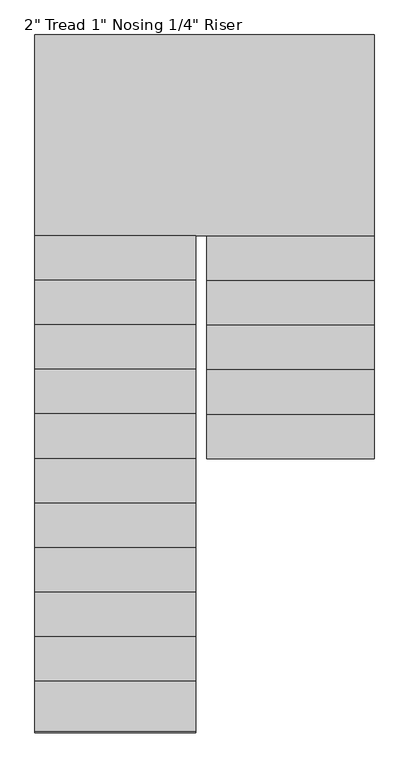
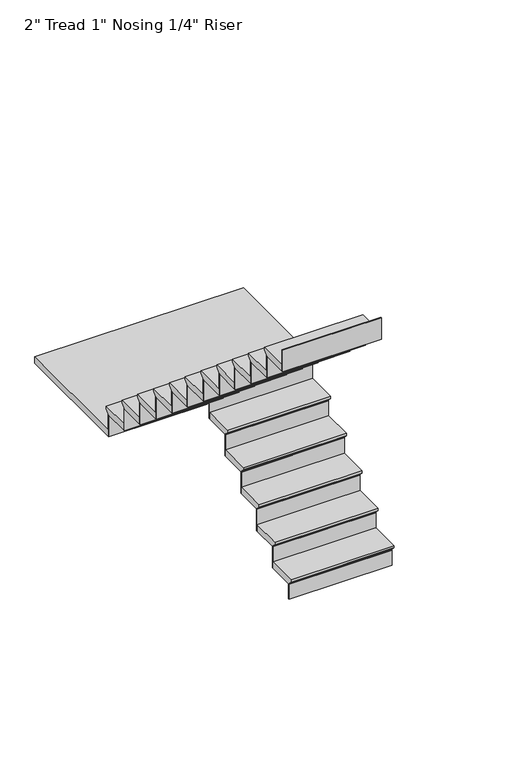
"""IFC4 building model written with IfcOpenShell, lengths in millimetres: stair flight geometry."""

from ifc_helpers import new_model, si_unit, origin, place, context, project, spatial, faceted_brep, source, transform, mapped, element, save


def stair_flight_e7bd6350(model_context):
    return source(origin(), model_context, "Body", "Brep", [
        faceted_brep([(-3749.597125, 2714.6319226, 30477.8833333), (-3749.597125, 2714.6319226, 30496.9333333), (-4512.2136682, 2714.6319226, 30496.9333333), (-4512.2136682, 2714.6319226, 30477.8833333), (-3749.597125, 2740.0319226, 30452.4833333), (-4512.2136682, 2740.0319226, 30452.4833333), (-3749.597125, 2943.2319226, 30496.9333333), (-4512.2136682, 2943.2319226, 30496.9333333), (-4512.2136682, 2740.0319226, 30446.1333333), (-4512.2136682, 2943.2319226, 30446.1333333), (-3749.597125, 2943.2319226, 30446.1333333), (-3749.597125, 2740.0319226, 30446.1333333)], [[[0, 1, 2, 3]], [[4, 0, 3, 5]], [[2, 1, 6, 7]], [[8, 9, 10, 11]], [[2, 7, 9, 8, 5, 3]], [[8, 11, 4, 5]], [[6, 1, 0, 4, 11, 10]], [[7, 6, 10, 9]]]),
        faceted_brep([(-3749.597125, 2740.0319226, 30446.1333333), (-3749.597125, 2740.0319226, 30327.6), (-3749.597125, 2746.3819226, 30327.6), (-3749.597125, 2746.3819226, 30446.1333333), (-4512.2136682, 2740.0319226, 30446.1333333), (-4512.2136682, 2746.3819226, 30446.1333333), (-4512.2136682, 2746.3819226, 30327.6), (-4512.2136682, 2740.0319226, 30327.6)], [[[0, 1, 2, 3]], [[4, 5, 6, 7]], [[1, 0, 4, 7]], [[2, 1, 7, 6]], [[3, 2, 6, 5]], [[0, 3, 5, 4]]]),
        faceted_brep([(-3749.597125, 2943.2319226, 30615.4666667), (-3749.597125, 2943.2319226, 30446.1333333), (-3749.597125, 2949.5819226, 30446.1333333), (-3749.597125, 2949.5819226, 30615.4666667), (-4512.2136682, 2943.2319226, 30615.4666667), (-4512.2136682, 2949.5819226, 30615.4666667), (-4512.2136682, 2949.5819226, 30446.1333333), (-4512.2136682, 2943.2319226, 30446.1333333)], [[[0, 1, 2, 3]], [[4, 5, 6, 7]], [[1, 0, 4, 7]], [[2, 1, 7, 6]], [[3, 2, 6, 5]], [[0, 3, 5, 4]]]),
        faceted_brep([(-4512.2136682, 2917.8319226, 30666.2666667), (-3749.597125, 2917.8319226, 30666.2666667), (-3749.597125, 3146.4319226, 30666.2666667), (-4512.2136682, 3146.4319226, 30666.2666667), (-4512.2136682, 2943.2319226, 30615.4666667), (-4512.2136682, 3146.4319226, 30615.4666667), (-3749.597125, 3146.4319226, 30615.4666667), (-3749.597125, 2943.2319226, 30615.4666667), (-4512.2136682, 2943.2319226, 30621.8166667), (-4512.2136682, 2917.8319226, 30647.2166667), (-3749.597125, 2943.2319226, 30621.8166667), (-3749.597125, 2917.8319226, 30647.2166667)], [[[0, 1, 2, 3]], [[4, 5, 6, 7]], [[0, 3, 5, 4, 8, 9]], [[4, 7, 10, 8]], [[2, 1, 11, 10, 7, 6]], [[3, 2, 6, 5]], [[11, 1, 0, 9]], [[10, 11, 9, 8]]]),
        faceted_brep([(-3749.597125, 3146.4319226, 30784.8), (-3749.597125, 3146.4319226, 30615.4666667), (-3749.597125, 3152.7819226, 30615.4666667), (-3749.597125, 3152.7819226, 30784.8), (-4512.2136682, 3146.4319226, 30784.8), (-4512.2136682, 3152.7819226, 30784.8), (-4512.2136682, 3152.7819226, 30615.4666667), (-4512.2136682, 3146.4319226, 30615.4666667)], [[[0, 1, 2, 3]], [[4, 5, 6, 7]], [[1, 0, 4, 7]], [[2, 1, 7, 6]], [[3, 2, 6, 5]], [[0, 3, 5, 4]]]),
        faceted_brep([(-4512.2136682, 3121.0319226, 30835.6), (-3749.597125, 3121.0319226, 30835.6), (-3749.597125, 3349.6319226, 30835.6), (-4512.2136682, 3349.6319226, 30835.6), (-4512.2136682, 3146.4319226, 30784.8), (-4512.2136682, 3349.6319226, 30784.8), (-3749.597125, 3349.6319226, 30784.8), (-3749.597125, 3146.4319226, 30784.8), (-4512.2136682, 3146.4319226, 30791.15), (-4512.2136682, 3121.0319226, 30816.55), (-3749.597125, 3146.4319226, 30791.15), (-3749.597125, 3121.0319226, 30816.55)], [[[0, 1, 2, 3]], [[4, 5, 6, 7]], [[0, 3, 5, 4, 8, 9]], [[4, 7, 10, 8]], [[2, 1, 11, 10, 7, 6]], [[3, 2, 6, 5]], [[11, 1, 0, 9]], [[10, 11, 9, 8]]]),
        faceted_brep([(-3749.597125, 3349.6319226, 30954.1333333), (-3749.597125, 3349.6319226, 30784.8), (-3749.597125, 3355.9819226, 30784.8), (-3749.597125, 3355.9819226, 30954.1333333), (-4512.2136682, 3349.6319226, 30954.1333333), (-4512.2136682, 3355.9819226, 30954.1333333), (-4512.2136682, 3355.9819226, 30784.8), (-4512.2136682, 3349.6319226, 30784.8)], [[[0, 1, 2, 3]], [[4, 5, 6, 7]], [[1, 0, 4, 7]], [[2, 1, 7, 6]], [[3, 2, 6, 5]], [[0, 3, 5, 4]]]),
        faceted_brep([(-4512.2136682, 3324.2319226, 31004.9333333), (-3749.597125, 3324.2319226, 31004.9333333), (-3749.597125, 3552.8319226, 31004.9333333), (-4512.2136682, 3552.8319226, 31004.9333333), (-4512.2136682, 3349.6319226, 30954.1333333), (-4512.2136682, 3552.8319226, 30954.1333333), (-3749.597125, 3552.8319226, 30954.1333333), (-3749.597125, 3349.6319226, 30954.1333333), (-4512.2136682, 3349.6319226, 30960.4833333), (-4512.2136682, 3324.2319226, 30985.8833333), (-3749.597125, 3349.6319226, 30960.4833333), (-3749.597125, 3324.2319226, 30985.8833333)], [[[0, 1, 2, 3]], [[4, 5, 6, 7]], [[0, 3, 5, 4, 8, 9]], [[4, 7, 10, 8]], [[2, 1, 11, 10, 7, 6]], [[3, 2, 6, 5]], [[11, 1, 0, 9]], [[10, 11, 9, 8]]]),
        faceted_brep([(-3749.597125, 3552.8319226, 31123.4666667), (-3749.597125, 3552.8319226, 30954.1333333), (-3749.597125, 3559.1819226, 30954.1333333), (-3749.597125, 3559.1819226, 31123.4666667), (-4512.2136682, 3552.8319226, 31123.4666667), (-4512.2136682, 3559.1819226, 31123.4666667), (-4512.2136682, 3559.1819226, 30954.1333333), (-4512.2136682, 3552.8319226, 30954.1333333)], [[[0, 1, 2, 3]], [[4, 5, 6, 7]], [[1, 0, 4, 7]], [[2, 1, 7, 6]], [[3, 2, 6, 5]], [[0, 3, 5, 4]]]),
        faceted_brep([(-4512.2136682, 3527.4319226, 31174.2666667), (-3749.597125, 3527.4319226, 31174.2666667), (-3749.597125, 3756.0319226, 31174.2666667), (-4512.2136682, 3756.0319226, 31174.2666667), (-4512.2136682, 3552.8319226, 31123.4666667), (-4512.2136682, 3756.0319226, 31123.4666667), (-3749.597125, 3756.0319226, 31123.4666667), (-3749.597125, 3552.8319226, 31123.4666667), (-4512.2136682, 3552.8319226, 31129.8166667), (-4512.2136682, 3527.4319226, 31155.2166667), (-3749.597125, 3552.8319226, 31129.8166667), (-3749.597125, 3527.4319226, 31155.2166667)], [[[0, 1, 2, 3]], [[4, 5, 6, 7]], [[0, 3, 5, 4, 8, 9]], [[4, 7, 10, 8]], [[2, 1, 11, 10, 7, 6]], [[3, 2, 6, 5]], [[11, 1, 0, 9]], [[10, 11, 9, 8]]]),
        faceted_brep([(-3749.597125, 3756.0319226, 31292.8), (-3749.597125, 3756.0319226, 31123.4666667), (-3749.597125, 3762.3819226, 31123.4666667), (-3749.597125, 3762.3819226, 31292.8), (-4512.2136682, 3756.0319226, 31292.8), (-4512.2136682, 3762.3819226, 31292.8), (-4512.2136682, 3762.3819226, 31123.4666667), (-4512.2136682, 3756.0319226, 31123.4666667)], [[[0, 1, 2, 3]], [[4, 5, 6, 7]], [[1, 0, 4, 7]], [[2, 1, 7, 6]], [[3, 2, 6, 5]], [[0, 3, 5, 4]]]),
        faceted_brep([(-4563.0136682, 3705.2319226, 31343.6), (-4563.0136682, 3730.6319226, 31343.6), (-3749.597125, 3730.6319226, 31343.6), (-3749.597125, 4645.0319226, 31343.6), (-5295.0246464, 4645.0319226, 31343.6), (-5295.0246464, 3705.2319226, 31343.6), (-4563.0136682, 3730.6319226, 31292.8), (-4563.0136682, 3705.2319226, 31292.8), (-5295.0246464, 3705.2319226, 31292.8), (-5295.0246464, 4645.0319226, 31292.8), (-3749.597125, 4645.0319226, 31292.8), (-3749.597125, 3756.0319226, 31292.8), (-4512.2136682, 3756.0319226, 31292.8), (-4512.2136682, 3730.6319226, 31292.8), (-4512.2136682, 3730.6319226, 31324.55), (-3749.597125, 3730.6319226, 31324.55), (-4512.2136682, 3756.0319226, 31299.15), (-3749.597125, 3756.0319226, 31299.15)], [[[0, 1, 2, 3, 4, 5]], [[6, 7, 8, 9, 10, 11, 12, 13]], [[1, 0, 7, 6]], [[2, 1, 6, 13, 14, 15]], [[13, 12, 16, 14]], [[12, 11, 17, 16]], [[3, 2, 15, 17, 11, 10]], [[4, 3, 10, 9]], [[5, 4, 9, 8]], [[0, 5, 8, 7]], [[17, 15, 14, 16]]]),
        faceted_brep([(-5295.0246464, 3705.2319226, 31462.1333333), (-5295.0246464, 3705.2319226, 31292.8), (-5295.0246464, 3698.8819226, 31292.8), (-5295.0246464, 3698.8819226, 31462.1333333), (-4563.0136682, 3705.2319226, 31462.1333333), (-4563.0136682, 3698.8819226, 31462.1333333), (-4563.0136682, 3698.8819226, 31292.8), (-4563.0136682, 3705.2319226, 31292.8)], [[[0, 1, 2, 3]], [[4, 5, 6, 7]], [[1, 0, 4, 7]], [[2, 1, 7, 6]], [[3, 2, 6, 5]], [[0, 3, 5, 4]]]),
        faceted_brep([(-4563.0136682, 3730.6319226, 31512.9333333), (-5295.0246464, 3730.6319226, 31512.9333333), (-5295.0246464, 3502.0319226, 31512.9333333), (-4563.0136682, 3502.0319226, 31512.9333333), (-4563.0136682, 3705.2319226, 31462.1333333), (-4563.0136682, 3502.0319226, 31462.1333333), (-5295.0246464, 3502.0319226, 31462.1333333), (-5295.0246464, 3705.2319226, 31462.1333333), (-4563.0136682, 3705.2319226, 31468.4833333), (-4563.0136682, 3730.6319226, 31493.8833333), (-5295.0246464, 3705.2319226, 31468.4833333), (-5295.0246464, 3730.6319226, 31493.8833333)], [[[0, 1, 2, 3]], [[4, 5, 6, 7]], [[0, 3, 5, 4, 8, 9]], [[4, 7, 10, 8]], [[2, 1, 11, 10, 7, 6]], [[3, 2, 6, 5]], [[11, 1, 0, 9]], [[10, 11, 9, 8]]]),
        faceted_brep([(-5295.0246464, 3502.0319226, 31631.4666667), (-5295.0246464, 3502.0319226, 31462.1333333), (-5295.0246464, 3495.6819226, 31462.1333333), (-5295.0246464, 3495.6819226, 31631.4666667), (-4563.0136682, 3502.0319226, 31631.4666667), (-4563.0136682, 3495.6819226, 31631.4666667), (-4563.0136682, 3495.6819226, 31462.1333333), (-4563.0136682, 3502.0319226, 31462.1333333)], [[[0, 1, 2, 3]], [[4, 5, 6, 7]], [[1, 0, 4, 7]], [[2, 1, 7, 6]], [[3, 2, 6, 5]], [[0, 3, 5, 4]]]),
        faceted_brep([(-4563.0136682, 3527.4319226, 31682.2666667), (-5295.0246464, 3527.4319226, 31682.2666667), (-5295.0246464, 3298.8319226, 31682.2666667), (-4563.0136682, 3298.8319226, 31682.2666667), (-4563.0136682, 3502.0319226, 31631.4666667), (-4563.0136682, 3298.8319226, 31631.4666667), (-5295.0246464, 3298.8319226, 31631.4666667), (-5295.0246464, 3502.0319226, 31631.4666667), (-4563.0136682, 3502.0319226, 31637.8166667), (-4563.0136682, 3527.4319226, 31663.2166667), (-5295.0246464, 3502.0319226, 31637.8166667), (-5295.0246464, 3527.4319226, 31663.2166667)], [[[0, 1, 2, 3]], [[4, 5, 6, 7]], [[0, 3, 5, 4, 8, 9]], [[4, 7, 10, 8]], [[2, 1, 11, 10, 7, 6]], [[3, 2, 6, 5]], [[11, 1, 0, 9]], [[10, 11, 9, 8]]]),
        faceted_brep([(-5295.0246464, 3298.8319226, 31800.8), (-5295.0246464, 3298.8319226, 31631.4666667), (-5295.0246464, 3292.4819226, 31631.4666667), (-5295.0246464, 3292.4819226, 31800.8), (-4563.0136682, 3298.8319226, 31800.8), (-4563.0136682, 3292.4819226, 31800.8), (-4563.0136682, 3292.4819226, 31631.4666667), (-4563.0136682, 3298.8319226, 31631.4666667)], [[[0, 1, 2, 3]], [[4, 5, 6, 7]], [[1, 0, 4, 7]], [[2, 1, 7, 6]], [[3, 2, 6, 5]], [[0, 3, 5, 4]]]),
        faceted_brep([(-4563.0136682, 3324.2319226, 31851.6), (-5295.0246464, 3324.2319226, 31851.6), (-5295.0246464, 3095.6319226, 31851.6), (-4563.0136682, 3095.6319226, 31851.6), (-4563.0136682, 3298.8319226, 31800.8), (-4563.0136682, 3095.6319226, 31800.8), (-5295.0246464, 3095.6319226, 31800.8), (-5295.0246464, 3298.8319226, 31800.8), (-4563.0136682, 3298.8319226, 31807.15), (-4563.0136682, 3324.2319226, 31832.55), (-5295.0246464, 3298.8319226, 31807.15), (-5295.0246464, 3324.2319226, 31832.55)], [[[0, 1, 2, 3]], [[4, 5, 6, 7]], [[0, 3, 5, 4, 8, 9]], [[4, 7, 10, 8]], [[2, 1, 11, 10, 7, 6]], [[3, 2, 6, 5]], [[11, 1, 0, 9]], [[10, 11, 9, 8]]]),
        faceted_brep([(-5295.0246464, 3095.6319226, 31970.1333333), (-5295.0246464, 3095.6319226, 31800.8), (-5295.0246464, 3089.2819226, 31800.8), (-5295.0246464, 3089.2819226, 31970.1333333), (-4563.0136682, 3095.6319226, 31970.1333333), (-4563.0136682, 3089.2819226, 31970.1333333), (-4563.0136682, 3089.2819226, 31800.8), (-4563.0136682, 3095.6319226, 31800.8)], [[[0, 1, 2, 3]], [[4, 5, 6, 7]], [[1, 0, 4, 7]], [[2, 1, 7, 6]], [[3, 2, 6, 5]], [[0, 3, 5, 4]]]),
        faceted_brep([(-4563.0136682, 3121.0319226, 32020.9333333), (-5295.0246464, 3121.0319226, 32020.9333333), (-5295.0246464, 2892.4319226, 32020.9333333), (-4563.0136682, 2892.4319226, 32020.9333333), (-4563.0136682, 3095.6319226, 31970.1333333), (-4563.0136682, 2892.4319226, 31970.1333333), (-5295.0246464, 2892.4319226, 31970.1333333), (-5295.0246464, 3095.6319226, 31970.1333333), (-4563.0136682, 3095.6319226, 31976.4833333), (-4563.0136682, 3121.0319226, 32001.8833333), (-5295.0246464, 3095.6319226, 31976.4833333), (-5295.0246464, 3121.0319226, 32001.8833333)], [[[0, 1, 2, 3]], [[4, 5, 6, 7]], [[0, 3, 5, 4, 8, 9]], [[4, 7, 10, 8]], [[2, 1, 11, 10, 7, 6]], [[3, 2, 6, 5]], [[11, 1, 0, 9]], [[10, 11, 9, 8]]]),
        faceted_brep([(-5295.0246464, 2892.4319226, 32139.4666667), (-5295.0246464, 2892.4319226, 31970.1333333), (-5295.0246464, 2886.0819226, 31970.1333333), (-5295.0246464, 2886.0819226, 32139.4666667), (-4563.0136682, 2892.4319226, 32139.4666667), (-4563.0136682, 2886.0819226, 32139.4666667), (-4563.0136682, 2886.0819226, 31970.1333333), (-4563.0136682, 2892.4319226, 31970.1333333)], [[[0, 1, 2, 3]], [[4, 5, 6, 7]], [[1, 0, 4, 7]], [[2, 1, 7, 6]], [[3, 2, 6, 5]], [[0, 3, 5, 4]]]),
        faceted_brep([(-4563.0136682, 2917.8319226, 32190.2666667), (-5295.0246464, 2917.8319226, 32190.2666667), (-5295.0246464, 2689.2319226, 32190.2666667), (-4563.0136682, 2689.2319226, 32190.2666667), (-4563.0136682, 2892.4319226, 32139.4666667), (-4563.0136682, 2689.2319226, 32139.4666667), (-5295.0246464, 2689.2319226, 32139.4666667), (-5295.0246464, 2892.4319226, 32139.4666667), (-4563.0136682, 2892.4319226, 32145.8166667), (-4563.0136682, 2917.8319226, 32171.2166667), (-5295.0246464, 2892.4319226, 32145.8166667), (-5295.0246464, 2917.8319226, 32171.2166667)], [[[0, 1, 2, 3]], [[4, 5, 6, 7]], [[0, 3, 5, 4, 8, 9]], [[4, 7, 10, 8]], [[2, 1, 11, 10, 7, 6]], [[3, 2, 6, 5]], [[11, 1, 0, 9]], [[10, 11, 9, 8]]]),
        faceted_brep([(-5295.0246464, 2689.2319226, 32308.8), (-5295.0246464, 2689.2319226, 32139.4666667), (-5295.0246464, 2682.8819226, 32139.4666667), (-5295.0246464, 2682.8819226, 32308.8), (-4563.0136682, 2689.2319226, 32308.8), (-4563.0136682, 2682.8819226, 32308.8), (-4563.0136682, 2682.8819226, 32139.4666667), (-4563.0136682, 2689.2319226, 32139.4666667)], [[[0, 1, 2, 3]], [[4, 5, 6, 7]], [[1, 0, 4, 7]], [[2, 1, 7, 6]], [[3, 2, 6, 5]], [[0, 3, 5, 4]]]),
        faceted_brep([(-4563.0136682, 2714.6319226, 32359.6), (-5295.0246464, 2714.6319226, 32359.6), (-5295.0246464, 2486.0319226, 32359.6), (-4563.0136682, 2486.0319226, 32359.6), (-4563.0136682, 2689.2319226, 32308.8), (-4563.0136682, 2486.0319226, 32308.8), (-5295.0246464, 2486.0319226, 32308.8), (-5295.0246464, 2689.2319226, 32308.8), (-4563.0136682, 2689.2319226, 32315.15), (-4563.0136682, 2714.6319226, 32340.55), (-5295.0246464, 2689.2319226, 32315.15), (-5295.0246464, 2714.6319226, 32340.55)], [[[0, 1, 2, 3]], [[4, 5, 6, 7]], [[0, 3, 5, 4, 8, 9]], [[4, 7, 10, 8]], [[2, 1, 11, 10, 7, 6]], [[3, 2, 6, 5]], [[11, 1, 0, 9]], [[10, 11, 9, 8]]]),
        faceted_brep([(-5295.0246464, 2486.0319226, 32478.1333333), (-5295.0246464, 2486.0319226, 32308.8), (-5295.0246464, 2479.6819226, 32308.8), (-5295.0246464, 2479.6819226, 32478.1333333), (-4563.0136682, 2486.0319226, 32478.1333333), (-4563.0136682, 2479.6819226, 32478.1333333), (-4563.0136682, 2479.6819226, 32308.8), (-4563.0136682, 2486.0319226, 32308.8)], [[[0, 1, 2, 3]], [[4, 5, 6, 7]], [[1, 0, 4, 7]], [[2, 1, 7, 6]], [[3, 2, 6, 5]], [[0, 3, 5, 4]]]),
        faceted_brep([(-4563.0136682, 2511.4319226, 32528.9333333), (-5295.0246464, 2511.4319226, 32528.9333333), (-5295.0246464, 2282.8319226, 32528.9333333), (-4563.0136682, 2282.8319226, 32528.9333333), (-4563.0136682, 2486.0319226, 32478.1333333), (-4563.0136682, 2282.8319226, 32478.1333333), (-5295.0246464, 2282.8319226, 32478.1333333), (-5295.0246464, 2486.0319226, 32478.1333333), (-4563.0136682, 2486.0319226, 32484.4833333), (-4563.0136682, 2511.4319226, 32509.8833333), (-5295.0246464, 2486.0319226, 32484.4833333), (-5295.0246464, 2511.4319226, 32509.8833333)], [[[0, 1, 2, 3]], [[4, 5, 6, 7]], [[0, 3, 5, 4, 8, 9]], [[4, 7, 10, 8]], [[2, 1, 11, 10, 7, 6]], [[3, 2, 6, 5]], [[11, 1, 0, 9]], [[10, 11, 9, 8]]]),
        faceted_brep([(-5295.0246464, 2282.8319226, 32647.4666667), (-5295.0246464, 2282.8319226, 32478.1333333), (-5295.0246464, 2276.4819226, 32478.1333333), (-5295.0246464, 2276.4819226, 32647.4666667), (-4563.0136682, 2282.8319226, 32647.4666667), (-4563.0136682, 2276.4819226, 32647.4666667), (-4563.0136682, 2276.4819226, 32478.1333333), (-4563.0136682, 2282.8319226, 32478.1333333)], [[[0, 1, 2, 3]], [[4, 5, 6, 7]], [[1, 0, 4, 7]], [[2, 1, 7, 6]], [[3, 2, 6, 5]], [[0, 3, 5, 4]]]),
        faceted_brep([(-4563.0136682, 2308.2319226, 32698.2666667), (-5295.0246464, 2308.2319226, 32698.2666667), (-5295.0246464, 2079.6319226, 32698.2666667), (-4563.0136682, 2079.6319226, 32698.2666667), (-4563.0136682, 2282.8319226, 32647.4666667), (-4563.0136682, 2079.6319226, 32647.4666667), (-5295.0246464, 2079.6319226, 32647.4666667), (-5295.0246464, 2282.8319226, 32647.4666667), (-4563.0136682, 2282.8319226, 32653.8166667), (-4563.0136682, 2308.2319226, 32679.2166667), (-5295.0246464, 2282.8319226, 32653.8166667), (-5295.0246464, 2308.2319226, 32679.2166667)], [[[0, 1, 2, 3]], [[4, 5, 6, 7]], [[0, 3, 5, 4, 8, 9]], [[4, 7, 10, 8]], [[2, 1, 11, 10, 7, 6]], [[3, 2, 6, 5]], [[11, 1, 0, 9]], [[10, 11, 9, 8]]]),
        faceted_brep([(-5295.0246464, 2079.6319226, 32816.8), (-5295.0246464, 2079.6319226, 32647.4666667), (-5295.0246464, 2073.2819226, 32647.4666667), (-5295.0246464, 2073.2819226, 32816.8), (-4563.0136682, 2079.6319226, 32816.8), (-4563.0136682, 2073.2819226, 32816.8), (-4563.0136682, 2073.2819226, 32647.4666667), (-4563.0136682, 2079.6319226, 32647.4666667)], [[[0, 1, 2, 3]], [[4, 5, 6, 7]], [[1, 0, 4, 7]], [[2, 1, 7, 6]], [[3, 2, 6, 5]], [[0, 3, 5, 4]]]),
        faceted_brep([(-4563.0136682, 2105.0319226, 32867.6), (-5295.0246464, 2105.0319226, 32867.6), (-5295.0246464, 1876.4319226, 32867.6), (-4563.0136682, 1876.4319226, 32867.6), (-4563.0136682, 2079.6319226, 32816.8), (-4563.0136682, 1876.4319226, 32816.8), (-5295.0246464, 1876.4319226, 32816.8), (-5295.0246464, 2079.6319226, 32816.8), (-4563.0136682, 2079.6319226, 32823.15), (-4563.0136682, 2105.0319226, 32848.55), (-5295.0246464, 2079.6319226, 32823.15), (-5295.0246464, 2105.0319226, 32848.55)], [[[0, 1, 2, 3]], [[4, 5, 6, 7]], [[0, 3, 5, 4, 8, 9]], [[4, 7, 10, 8]], [[2, 1, 11, 10, 7, 6]], [[3, 2, 6, 5]], [[11, 1, 0, 9]], [[10, 11, 9, 8]]]),
        faceted_brep([(-5295.0246464, 1876.4319226, 32986.1333333), (-5295.0246464, 1876.4319226, 32816.8), (-5295.0246464, 1870.0819226, 32816.8), (-5295.0246464, 1870.0819226, 32986.1333333), (-4563.0136682, 1876.4319226, 32986.1333333), (-4563.0136682, 1870.0819226, 32986.1333333), (-4563.0136682, 1870.0819226, 32816.8), (-4563.0136682, 1876.4319226, 32816.8)], [[[0, 1, 2, 3]], [[4, 5, 6, 7]], [[1, 0, 4, 7]], [[2, 1, 7, 6]], [[3, 2, 6, 5]], [[0, 3, 5, 4]]]),
        faceted_brep([(-4563.0136682, 1901.8319226, 33036.9333333), (-5295.0246464, 1901.8319226, 33036.9333333), (-5295.0246464, 1673.2319226, 33036.9333333), (-4563.0136682, 1673.2319226, 33036.9333333), (-4563.0136682, 1876.4319226, 32986.1333333), (-4563.0136682, 1673.2319226, 32986.1333333), (-5295.0246464, 1673.2319226, 32986.1333333), (-5295.0246464, 1876.4319226, 32986.1333333), (-4563.0136682, 1876.4319226, 32992.4833333), (-4563.0136682, 1901.8319226, 33017.8833333), (-5295.0246464, 1876.4319226, 32992.4833333), (-5295.0246464, 1901.8319226, 33017.8833333)], [[[0, 1, 2, 3]], [[4, 5, 6, 7]], [[0, 3, 5, 4, 8, 9]], [[4, 7, 10, 8]], [[2, 1, 11, 10, 7, 6]], [[3, 2, 6, 5]], [[11, 1, 0, 9]], [[10, 11, 9, 8]]]),
        faceted_brep([(-5295.0246464, 1673.2319226, 33155.4666667), (-5295.0246464, 1673.2319226, 32986.1333333), (-5295.0246464, 1666.8819226, 32986.1333333), (-5295.0246464, 1666.8819226, 33155.4666667), (-4563.0136682, 1673.2319226, 33155.4666667), (-4563.0136682, 1666.8819226, 33155.4666667), (-4563.0136682, 1666.8819226, 32986.1333333), (-4563.0136682, 1673.2319226, 32986.1333333)], [[[0, 1, 2, 3]], [[4, 5, 6, 7]], [[1, 0, 4, 7]], [[2, 1, 7, 6]], [[3, 2, 6, 5]], [[0, 3, 5, 4]]]),
        faceted_brep([(-4563.0136682, 1698.6319226, 33206.2666667), (-5295.0246464, 1698.6319226, 33206.2666667), (-5295.0246464, 1470.0319226, 33206.2666667), (-4563.0136682, 1470.0319226, 33206.2666667), (-4563.0136682, 1673.2319226, 33155.4666667), (-4563.0136682, 1470.0319226, 33155.4666667), (-5295.0246464, 1470.0319226, 33155.4666667), (-5295.0246464, 1673.2319226, 33155.4666667), (-4563.0136682, 1673.2319226, 33161.8166667), (-4563.0136682, 1698.6319226, 33187.2166667), (-5295.0246464, 1673.2319226, 33161.8166667), (-5295.0246464, 1698.6319226, 33187.2166667)], [[[0, 1, 2, 3]], [[4, 5, 6, 7]], [[0, 3, 5, 4, 8, 9]], [[4, 7, 10, 8]], [[2, 1, 11, 10, 7, 6]], [[3, 2, 6, 5]], [[11, 1, 0, 9]], [[10, 11, 9, 8]]]),
        faceted_brep([(-5295.0246464, 1470.0319226, 33324.8), (-5295.0246464, 1470.0319226, 33155.4666667), (-5295.0246464, 1463.6819226, 33155.4666667), (-5295.0246464, 1463.6819226, 33324.8), (-4563.0136682, 1470.0319226, 33324.8), (-4563.0136682, 1463.6819226, 33324.8), (-4563.0136682, 1463.6819226, 33155.4666667), (-4563.0136682, 1470.0319226, 33155.4666667)], [[[0, 1, 2, 3]], [[4, 5, 6, 7]], [[1, 0, 4, 7]], [[2, 1, 7, 6]], [[3, 2, 6, 5]], [[0, 3, 5, 4]]]),
    ])


if __name__ == "__main__":
    model = new_model("IFC4")
    model_context = context("Model", 3, world=origin())
    ifc_project = project(units=[si_unit("LENGTHUNIT", "METRE", prefix="MILLI")], contexts=[model_context])
    site = spatial("IfcSite", under=ifc_project)
    building = spatial("IfcBuilding", under=site)
    placement = place(None, origin())
    stair_flight_shape = stair_flight_e7bd6350(model_context)
    element("IfcStairFlight", 1, ObjectType="2\" Tread 1\" Nosing 1/4\" Riser", at=placement, inside=building, context=model_context, shape_type="MappedRepresentation", body=[
        mapped(stair_flight_shape, transform((0.0, 0.0, 0.0), x_axis=(1.0, 0.0, 0.0), y_axis=(0.0, 1.0, 0.0), z_axis=(0.0, 0.0, 1.0))),
    ])
    save(model, "model.ifc")
